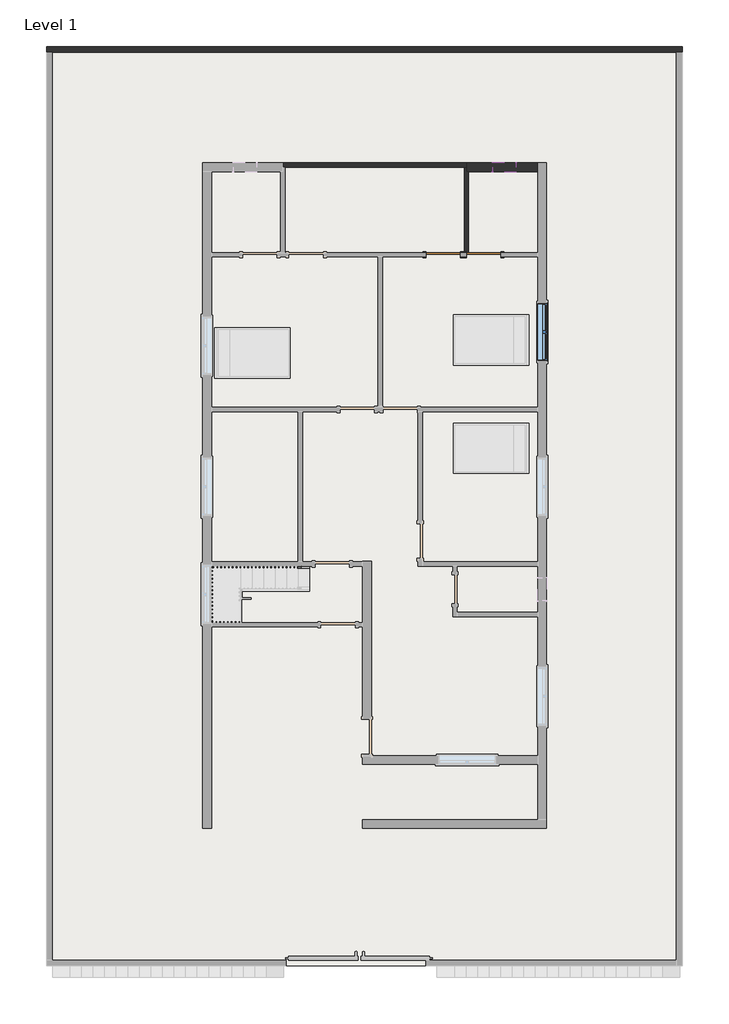
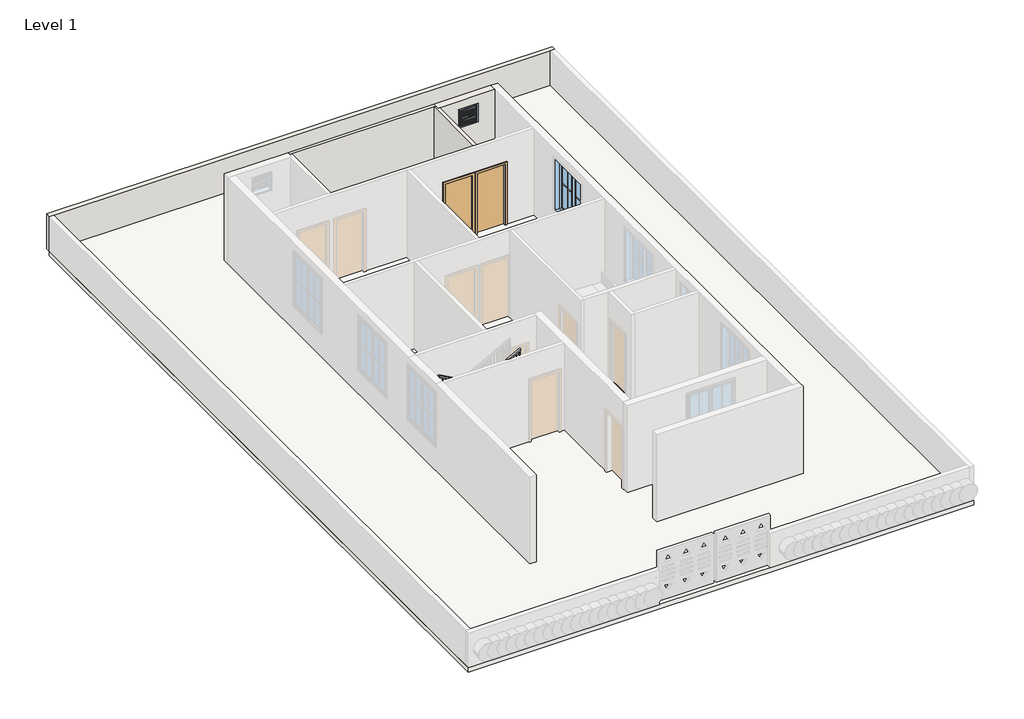
# One storey, part 2 of 3: 4 walls, 2 doors, 2 windows, 1 railing, 1 slab.
"""IFC4 building model written with IfcOpenShell, lengths in millimetres."""

from ifc_helpers import new_model, si_unit, frame, origin, origin_with_axes, place, context, project, spatial, polyline, outline, extrude, faceted_brep, transform, mapped, element, save
from components import single_flush_door_3_e5f9f3c4, single_flush_door_3_305aa2a5, window_casement_double_win_5_f93960c7, window_f2d8fef0

model = new_model("IFC4")

# Units and contexts
model_context = context("Model", 3, world=origin())
ifc_project = project(units=[si_unit("LENGTHUNIT", "METRE", prefix="MILLI")], contexts=[model_context])

# Site, building, storey
site = spatial("IfcSite", under=ifc_project)
building = spatial("IfcBuilding", under=site)
storey = spatial("IfcBuildingStorey", under=building, Name="Level 1", Elevation=0.0)

# Doors
placement = place(None, origin())
single_flush_door_3_shape = single_flush_door_3_e5f9f3c4(model_context)
element("IfcDoor", 1, ObjectType="Single-Flush : DOOR 3'", at=placement, inside=storey, context=model_context, shape_type="MappedRepresentation", body=[
    mapped(single_flush_door_3_shape, transform((555.4379845, 6040.5434309, 0.0), x_axis=(1.0, 0.0, 0.0), y_axis=(0.0, 1.0, 0.0), z_axis=(0.0, 0.0, 1.0))),
])
single_flush_door_3_2_shape = single_flush_door_3_305aa2a5(model_context)
element("IfcDoor", 2, ObjectType="Single-Flush : DOOR 3'", at=placement, inside=storey, context=model_context, shape_type="MappedRepresentation", body=[
    mapped(single_flush_door_3_2_shape, transform((1622.2379845, 6040.5434309, 0.0), x_axis=(-1.0, 0.0, 0.0), y_axis=(0.0, -1.0, 0.0), z_axis=(0.0, 0.0, 1.0))),
])

# Railing
element("IfcRailing", 3, ObjectType="Handrail - Rectangular", at=placement, inside=storey, context=model_context, shape_type="SolidModel", body=[
    faceted_brep([(-2968.8120155, -2220.8065691, 1083.7333333), (-2968.8120155, -2220.8065691, 1025.620221), (-2968.8120155, -2170.0065691, 1025.620221), (-2968.8120155, -2170.0065691, 1083.7333333), (-4797.6120155, -2220.8065691, 2099.7333333), (-4810.7756177, -2220.8065691, 2048.9333333), (-4810.7756177, -2170.0065691, 2048.9333333), (-4797.6120155, -2170.0065691, 2099.7333333), (-5508.8120155, -2220.8065691, 2099.7333333), (-5508.8120155, -2220.8065691, 2048.9333333), (-5559.6120155, -2170.0065691, 2048.9333333), (-5559.6120155, -2170.0065691, 2099.7333333), (-5508.8120155, -3624.1565691, 2099.7333333), (-5508.8120155, -3624.1565691, 2048.9333333), (-5559.6120155, -3674.9565691, 2048.9333333), (-5559.6120155, -3674.9565691, 2099.7333333), (-5102.4120155, -3624.1565691, 2099.7333333), (-5089.2484132, -3624.1565691, 2048.9333333), (-5089.2484132, -3674.9565691, 2048.9333333), (-5102.4120155, -3674.9565691, 2099.7333333), (-2968.8120155, -3624.1565691, 3285.0666667), (-2968.8120155, -3674.9565691, 3285.0666667), (-2968.8120155, -3674.9565691, 3226.9535543), (-2968.8120155, -3624.1565691, 3226.9535543)], [[[0, 1, 2, 3]], [[1, 0, 4, 5]], [[2, 1, 5, 6]], [[3, 2, 6, 7]], [[0, 3, 7, 4]], [[5, 4, 8, 9]], [[6, 5, 9, 10]], [[7, 6, 10, 11]], [[4, 7, 11, 8]], [[9, 8, 12, 13]], [[10, 9, 13, 14]], [[11, 10, 14, 15]], [[8, 11, 15, 12]], [[13, 12, 16, 17]], [[14, 13, 17, 18]], [[15, 14, 18, 19]], [[12, 15, 19, 16]], [[20, 21, 22, 23]], [[17, 16, 20, 23]], [[18, 17, 23, 22]], [[19, 18, 22, 21]], [[16, 19, 21, 20]]]),
    extrude(outline(polyline([(3218.1341099, -2984.6870155), (3207.5507765, -3003.7370155), (2201.3333333, -3003.7370155), (2201.3333333, -2984.6870155), (3218.1341099, -2984.6870155)])), frame((0.0, -3659.0815691, 0.0), z_axis=(0.0, 1.0, 0.0), x_axis=(0.0, 0.0, 1.0)), (0.0, 0.0, 1.0), 19.05),
    extrude(outline(polyline([(3161.6896654, -3086.2870155), (3151.1063321, -3105.3370155), (2201.3333333, -3105.3370155), (2201.3333333, -3086.2870155), (3161.6896654, -3086.2870155)])), frame((0.0, -3659.0815691, 0.0), z_axis=(0.0, 1.0, 0.0), x_axis=(0.0, 0.0, 1.0)), (0.0, 0.0, 1.0), 19.05),
    extrude(outline(polyline([(3105.245221, -3187.8870155), (3094.6618876, -3206.9370155), (2201.3333333, -3206.9370155), (2201.3333333, -3187.8870155), (3105.245221, -3187.8870155)])), frame((0.0, -3659.0815691, 0.0), z_axis=(0.0, 1.0, 0.0), x_axis=(0.0, 0.0, 1.0)), (0.0, 0.0, 1.0), 19.05),
    extrude(outline(polyline([(3048.8007765, -3289.4870155), (3038.2174432, -3308.5370155), (2032.0, -3308.5370155), (2032.0, -3289.4870155), (3048.8007765, -3289.4870155)])), frame((0.0, -3659.0815691, 0.0), z_axis=(0.0, 1.0, 0.0), x_axis=(0.0, 0.0, 1.0)), (0.0, 0.0, 1.0), 19.05),
    extrude(outline(polyline([(2992.3563321, -3391.0870155), (2981.7729988, -3410.1370155), (2032.0, -3410.1370155), (2032.0, -3391.0870155), (2992.3563321, -3391.0870155)])), frame((0.0, -3659.0815691, 0.0), z_axis=(0.0, 1.0, 0.0), x_axis=(0.0, 0.0, 1.0)), (0.0, 0.0, 1.0), 19.05),
    extrude(outline(polyline([(2935.9118876, -3492.6870155), (2925.3285543, -3511.7370155), (2032.0, -3511.7370155), (2032.0, -3492.6870155), (2935.9118876, -3492.6870155)])), frame((0.0, -3659.0815691, 0.0), z_axis=(0.0, 1.0, 0.0), x_axis=(0.0, 0.0, 1.0)), (0.0, 0.0, 1.0), 19.05),
    extrude(outline(polyline([(2879.4674432, -3594.2870155), (2868.8841099, -3613.3370155), (1862.6666667, -3613.3370155), (1862.6666667, -3594.2870155), (2879.4674432, -3594.2870155)])), frame((0.0, -3659.0815691, 0.0), z_axis=(0.0, 1.0, 0.0), x_axis=(0.0, 0.0, 1.0)), (0.0, 0.0, 1.0), 19.05),
    extrude(outline(polyline([(2823.0229988, -3695.8870155), (2812.4396654, -3714.9370155), (1862.6666667, -3714.9370155), (1862.6666667, -3695.8870155), (2823.0229988, -3695.8870155)])), frame((0.0, -3659.0815691, 0.0), z_axis=(0.0, 1.0, 0.0), x_axis=(0.0, 0.0, 1.0)), (0.0, 0.0, 1.0), 19.05),
    extrude(outline(polyline([(2766.5785543, -3797.4870155), (2755.995221, -3816.5370155), (1862.6666667, -3816.5370155), (1862.6666667, -3797.4870155), (2766.5785543, -3797.4870155)])), frame((0.0, -3659.0815691, 0.0), z_axis=(0.0, 1.0, 0.0), x_axis=(0.0, 0.0, 1.0)), (0.0, 0.0, 1.0), 19.05),
    extrude(outline(polyline([(2710.1341099, -3899.0870155), (2699.5507765, -3918.1370155), (1693.3333333, -3918.1370155), (1693.3333333, -3899.0870155), (2710.1341099, -3899.0870155)])), frame((0.0, -3659.0815691, 0.0), z_axis=(0.0, 1.0, 0.0), x_axis=(0.0, 0.0, 1.0)), (0.0, 0.0, 1.0), 19.05),
    extrude(outline(polyline([(2653.6896654, -4000.6870155), (2643.1063321, -4019.7370155), (1693.3333333, -4019.7370155), (1693.3333333, -4000.6870155), (2653.6896654, -4000.6870155)])), frame((0.0, -3659.0815691, 0.0), z_axis=(0.0, 1.0, 0.0), x_axis=(0.0, 0.0, 1.0)), (0.0, 0.0, 1.0), 19.05),
    extrude(outline(polyline([(2597.245221, -4102.2870155), (2586.6618876, -4121.3370155), (1693.3333333, -4121.3370155), (1693.3333333, -4102.2870155), (2597.245221, -4102.2870155)])), frame((0.0, -3659.0815691, 0.0), z_axis=(0.0, 1.0, 0.0), x_axis=(0.0, 0.0, 1.0)), (0.0, 0.0, 1.0), 19.05),
    extrude(outline(polyline([(2540.8007765, -4203.8870155), (2530.2174432, -4222.9370155), (1524.0, -4222.9370155), (1524.0, -4203.8870155), (2540.8007765, -4203.8870155)])), frame((0.0, -3659.0815691, 0.0), z_axis=(0.0, 1.0, 0.0), x_axis=(0.0, 0.0, 1.0)), (0.0, 0.0, 1.0), 19.05),
    extrude(outline(polyline([(2484.3563321, -4305.4870155), (2473.7729988, -4324.5370155), (1524.0, -4324.5370155), (1524.0, -4305.4870155), (2484.3563321, -4305.4870155)])), frame((0.0, -3659.0815691, 0.0), z_axis=(0.0, 1.0, 0.0), x_axis=(0.0, 0.0, 1.0)), (0.0, 0.0, 1.0), 19.05),
    extrude(outline(polyline([(2427.9118876, -4407.0870155), (2417.3285543, -4426.1370155), (1524.0, -4426.1370155), (1524.0, -4407.0870155), (2427.9118876, -4407.0870155)])), frame((0.0, -3659.0815691, 0.0), z_axis=(0.0, 1.0, 0.0), x_axis=(0.0, 0.0, 1.0)), (0.0, 0.0, 1.0), 19.05),
    extrude(outline(polyline([(2371.4674432, -4508.6870155), (2360.8841099, -4527.7370155), (1354.6666667, -4527.7370155), (1354.6666667, -4508.6870155), (2371.4674432, -4508.6870155)])), frame((0.0, -3659.0815691, 0.0), z_axis=(0.0, 1.0, 0.0), x_axis=(0.0, 0.0, 1.0)), (0.0, 0.0, 1.0), 19.05),
    extrude(outline(polyline([(2315.0229988, -4610.2870155), (2304.4396654, -4629.3370155), (1354.6666667, -4629.3370155), (1354.6666667, -4610.2870155), (2315.0229988, -4610.2870155)])), frame((0.0, -3659.0815691, 0.0), z_axis=(0.0, 1.0, 0.0), x_axis=(0.0, 0.0, 1.0)), (0.0, 0.0, 1.0), 19.05),
    extrude(outline(polyline([(2258.5785543, -4711.8870155), (2247.995221, -4730.9370155), (1354.6666667, -4730.9370155), (1354.6666667, -4711.8870155), (2258.5785543, -4711.8870155)])), frame((0.0, -3659.0815691, 0.0), z_axis=(0.0, 1.0, 0.0), x_axis=(0.0, 0.0, 1.0)), (0.0, 0.0, 1.0), 19.05),
    extrude(outline(polyline([(2202.1341099, -4813.4870155), (2191.5507765, -4832.5370155), (1185.3333333, -4832.5370155), (1185.3333333, -4813.4870155), (2202.1341099, -4813.4870155)])), frame((0.0, -3659.0815691, 0.0), z_axis=(0.0, 1.0, 0.0), x_axis=(0.0, 0.0, 1.0)), (0.0, 0.0, 1.0), 19.05),
    extrude(outline(polyline([(2145.6896654, -4915.0870155), (2135.1063321, -4934.1370155), (1185.3333333, -4934.1370155), (1185.3333333, -4915.0870155), (2145.6896654, -4915.0870155)])), frame((0.0, -3659.0815691, 0.0), z_axis=(0.0, 1.0, 0.0), x_axis=(0.0, 0.0, 1.0)), (0.0, 0.0, 1.0), 19.05),
    extrude(outline(polyline([(2089.245221, -5016.6870155), (2078.6618876, -5035.7370155), (1185.3333333, -5035.7370155), (1185.3333333, -5016.6870155), (2089.245221, -5016.6870155)])), frame((0.0, -3659.0815691, 0.0), z_axis=(0.0, 1.0, 0.0), x_axis=(0.0, 0.0, 1.0)), (0.0, 0.0, 1.0), 19.05),
    extrude(outline(polyline([(-5137.3370155, -3659.0815691), (-5137.3370155, -3640.0315691), (-5118.2870155, -3640.0315691), (-5118.2870155, -3659.0815691), (-5137.3370155, -3659.0815691)])), frame((0.0, 0.0, 1185.3333333), z_axis=(0.0, 0.0, 1.0), x_axis=(1.0, 0.0, 0.0)), (0.0, 0.0, 1.0), 863.6),
    extrude(outline(polyline([(-5238.9370155, -3659.0815691), (-5238.9370155, -3640.0315691), (-5219.8870155, -3640.0315691), (-5219.8870155, -3659.0815691), (-5238.9370155, -3659.0815691)])), frame((0.0, 0.0, 1185.3333333), z_axis=(0.0, 0.0, 1.0), x_axis=(1.0, 0.0, 0.0)), (0.0, 0.0, 1.0), 863.6),
    extrude(outline(polyline([(-5340.5370155, -3659.0815691), (-5340.5370155, -3640.0315691), (-5321.4870155, -3640.0315691), (-5321.4870155, -3659.0815691), (-5340.5370155, -3659.0815691)])), frame((0.0, 0.0, 1185.3333333), z_axis=(0.0, 0.0, 1.0), x_axis=(1.0, 0.0, 0.0)), (0.0, 0.0, 1.0), 863.6),
    extrude(outline(polyline([(-5442.1370155, -3659.0815691), (-5442.1370155, -3640.0315691), (-5423.0870155, -3640.0315691), (-5423.0870155, -3659.0815691), (-5442.1370155, -3659.0815691)])), frame((0.0, 0.0, 1185.3333333), z_axis=(0.0, 0.0, 1.0), x_axis=(1.0, 0.0, 0.0)), (0.0, 0.0, 1.0), 863.6),
    extrude(outline(polyline([(-5543.7370155, -3608.2815691), (-5524.6870155, -3608.2815691), (-5524.6870155, -3627.3315691), (-5543.7370155, -3627.3315691), (-5543.7370155, -3608.2815691)])), frame((0.0, 0.0, 1185.3333333), z_axis=(0.0, 0.0, 1.0), x_axis=(1.0, 0.0, 0.0)), (0.0, 0.0, 1.0), 863.6),
    extrude(outline(polyline([(-5543.7370155, -3506.6815691), (-5524.6870155, -3506.6815691), (-5524.6870155, -3525.7315691), (-5543.7370155, -3525.7315691), (-5543.7370155, -3506.6815691)])), frame((0.0, 0.0, 1185.3333333), z_axis=(0.0, 0.0, 1.0), x_axis=(1.0, 0.0, 0.0)), (0.0, 0.0, 1.0), 863.6),
    extrude(outline(polyline([(-5543.7370155, -3405.0815691), (-5524.6870155, -3405.0815691), (-5524.6870155, -3424.1315691), (-5543.7370155, -3424.1315691), (-5543.7370155, -3405.0815691)])), frame((0.0, 0.0, 1185.3333333), z_axis=(0.0, 0.0, 1.0), x_axis=(1.0, 0.0, 0.0)), (0.0, 0.0, 1.0), 863.6),
    extrude(outline(polyline([(-5543.7370155, -3303.4815691), (-5524.6870155, -3303.4815691), (-5524.6870155, -3322.5315691), (-5543.7370155, -3322.5315691), (-5543.7370155, -3303.4815691)])), frame((0.0, 0.0, 1185.3333333), z_axis=(0.0, 0.0, 1.0), x_axis=(1.0, 0.0, 0.0)), (0.0, 0.0, 1.0), 863.6),
    extrude(outline(polyline([(-5543.7370155, -3201.8815691), (-5524.6870155, -3201.8815691), (-5524.6870155, -3220.9315691), (-5543.7370155, -3220.9315691), (-5543.7370155, -3201.8815691)])), frame((0.0, 0.0, 1185.3333333), z_axis=(0.0, 0.0, 1.0), x_axis=(1.0, 0.0, 0.0)), (0.0, 0.0, 1.0), 863.6),
    extrude(outline(polyline([(-5543.7370155, -3100.2815691), (-5524.6870155, -3100.2815691), (-5524.6870155, -3119.3315691), (-5543.7370155, -3119.3315691), (-5543.7370155, -3100.2815691)])), frame((0.0, 0.0, 1185.3333333), z_axis=(0.0, 0.0, 1.0), x_axis=(1.0, 0.0, 0.0)), (0.0, 0.0, 1.0), 863.6),
    extrude(outline(polyline([(-5543.7370155, -2998.6815691), (-5524.6870155, -2998.6815691), (-5524.6870155, -3017.7315691), (-5543.7370155, -3017.7315691), (-5543.7370155, -2998.6815691)])), frame((0.0, 0.0, 1185.3333333), z_axis=(0.0, 0.0, 1.0), x_axis=(1.0, 0.0, 0.0)), (0.0, 0.0, 1.0), 863.6),
    extrude(outline(polyline([(-5543.7370155, -2897.0815691), (-5524.6870155, -2897.0815691), (-5524.6870155, -2916.1315691), (-5543.7370155, -2916.1315691), (-5543.7370155, -2897.0815691)])), frame((0.0, 0.0, 1185.3333333), z_axis=(0.0, 0.0, 1.0), x_axis=(1.0, 0.0, 0.0)), (0.0, 0.0, 1.0), 863.6),
    extrude(outline(polyline([(-5543.7370155, -2795.4815691), (-5524.6870155, -2795.4815691), (-5524.6870155, -2814.5315691), (-5543.7370155, -2814.5315691), (-5543.7370155, -2795.4815691)])), frame((0.0, 0.0, 1185.3333333), z_axis=(0.0, 0.0, 1.0), x_axis=(1.0, 0.0, 0.0)), (0.0, 0.0, 1.0), 863.6),
    extrude(outline(polyline([(-5543.7370155, -2693.8815691), (-5524.6870155, -2693.8815691), (-5524.6870155, -2712.9315691), (-5543.7370155, -2712.9315691), (-5543.7370155, -2693.8815691)])), frame((0.0, 0.0, 1185.3333333), z_axis=(0.0, 0.0, 1.0), x_axis=(1.0, 0.0, 0.0)), (0.0, 0.0, 1.0), 863.6),
    extrude(outline(polyline([(-5543.7370155, -2592.2815691), (-5524.6870155, -2592.2815691), (-5524.6870155, -2611.3315691), (-5543.7370155, -2611.3315691), (-5543.7370155, -2592.2815691)])), frame((0.0, 0.0, 1185.3333333), z_axis=(0.0, 0.0, 1.0), x_axis=(1.0, 0.0, 0.0)), (0.0, 0.0, 1.0), 863.6),
    extrude(outline(polyline([(-5543.7370155, -2490.6815691), (-5524.6870155, -2490.6815691), (-5524.6870155, -2509.7315691), (-5543.7370155, -2509.7315691), (-5543.7370155, -2490.6815691)])), frame((0.0, 0.0, 1185.3333333), z_axis=(0.0, 0.0, 1.0), x_axis=(1.0, 0.0, 0.0)), (0.0, 0.0, 1.0), 863.6),
    extrude(outline(polyline([(-5543.7370155, -2389.0815691), (-5524.6870155, -2389.0815691), (-5524.6870155, -2408.1315691), (-5543.7370155, -2408.1315691), (-5543.7370155, -2389.0815691)])), frame((0.0, 0.0, 1185.3333333), z_axis=(0.0, 0.0, 1.0), x_axis=(1.0, 0.0, 0.0)), (0.0, 0.0, 1.0), 863.6),
    extrude(outline(polyline([(-5543.7370155, -2287.4815691), (-5524.6870155, -2287.4815691), (-5524.6870155, -2306.5315691), (-5543.7370155, -2306.5315691), (-5543.7370155, -2287.4815691)])), frame((0.0, 0.0, 1185.3333333), z_axis=(0.0, 0.0, 1.0), x_axis=(1.0, 0.0, 0.0)), (0.0, 0.0, 1.0), 863.6),
    extrude(outline(polyline([(-5499.2870155, -2185.8815691), (-5499.2870155, -2204.9315691), (-5518.3370155, -2204.9315691), (-5518.3370155, -2185.8815691), (-5499.2870155, -2185.8815691)])), frame((0.0, 0.0, 1185.3333333), z_axis=(0.0, 0.0, 1.0), x_axis=(1.0, 0.0, 0.0)), (0.0, 0.0, 1.0), 863.6),
    extrude(outline(polyline([(-5397.6870155, -2185.8815691), (-5397.6870155, -2204.9315691), (-5416.7370155, -2204.9315691), (-5416.7370155, -2185.8815691), (-5397.6870155, -2185.8815691)])), frame((0.0, 0.0, 1185.3333333), z_axis=(0.0, 0.0, 1.0), x_axis=(1.0, 0.0, 0.0)), (0.0, 0.0, 1.0), 863.6),
    extrude(outline(polyline([(-5296.0870155, -2185.8815691), (-5296.0870155, -2204.9315691), (-5315.1370155, -2204.9315691), (-5315.1370155, -2185.8815691), (-5296.0870155, -2185.8815691)])), frame((0.0, 0.0, 1185.3333333), z_axis=(0.0, 0.0, 1.0), x_axis=(1.0, 0.0, 0.0)), (0.0, 0.0, 1.0), 863.6),
    extrude(outline(polyline([(-5194.4870155, -2185.8815691), (-5194.4870155, -2204.9315691), (-5213.5370155, -2204.9315691), (-5213.5370155, -2185.8815691), (-5194.4870155, -2185.8815691)])), frame((0.0, 0.0, 1185.3333333), z_axis=(0.0, 0.0, 1.0), x_axis=(1.0, 0.0, 0.0)), (0.0, 0.0, 1.0), 863.6),
    extrude(outline(polyline([(-5092.8870155, -2185.8815691), (-5092.8870155, -2204.9315691), (-5111.9370155, -2204.9315691), (-5111.9370155, -2185.8815691), (-5092.8870155, -2185.8815691)])), frame((0.0, 0.0, 1185.3333333), z_axis=(0.0, 0.0, 1.0), x_axis=(1.0, 0.0, 0.0)), (0.0, 0.0, 1.0), 863.6),
    extrude(outline(polyline([(-4991.2870155, -2185.8815691), (-4991.2870155, -2204.9315691), (-5010.3370155, -2204.9315691), (-5010.3370155, -2185.8815691), (-4991.2870155, -2185.8815691)])), frame((0.0, 0.0, 1185.3333333), z_axis=(0.0, 0.0, 1.0), x_axis=(1.0, 0.0, 0.0)), (0.0, 0.0, 1.0), 863.6),
    extrude(outline(polyline([(-4889.6870155, -2185.8815691), (-4889.6870155, -2204.9315691), (-4908.7370155, -2204.9315691), (-4908.7370155, -2185.8815691), (-4889.6870155, -2185.8815691)])), frame((0.0, 0.0, 1185.3333333), z_axis=(0.0, 0.0, 1.0), x_axis=(1.0, 0.0, 0.0)), (0.0, 0.0, 1.0), 863.6),
    extrude(outline(polyline([(2036.3285543, -4788.0870155), (2046.9118876, -4807.1370155), (1185.3333333, -4807.1370155), (1185.3333333, -4788.0870155), (2036.3285543, -4788.0870155)])), frame((0.0, -2204.9315691, 0.0), z_axis=(0.0, 1.0, 0.0), x_axis=(0.0, 0.0, 1.0)), (0.0, 0.0, 1.0), 19.05),
    extrude(outline(polyline([(1979.8841099, -4686.4870155), (1990.4674432, -4705.5370155), (1016.0, -4705.5370155), (1016.0, -4686.4870155), (1979.8841099, -4686.4870155)])), frame((0.0, -2204.9315691, 0.0), z_axis=(0.0, 1.0, 0.0), x_axis=(0.0, 0.0, 1.0)), (0.0, 0.0, 1.0), 19.05),
    extrude(outline(polyline([(1923.4396654, -4584.8870155), (1934.0229988, -4603.9370155), (1016.0, -4603.9370155), (1016.0, -4584.8870155), (1923.4396654, -4584.8870155)])), frame((0.0, -2204.9315691, 0.0), z_axis=(0.0, 1.0, 0.0), x_axis=(0.0, 0.0, 1.0)), (0.0, 0.0, 1.0), 19.05),
    extrude(outline(polyline([(1866.995221, -4483.2870155), (1877.5785543, -4502.3370155), (1016.0, -4502.3370155), (1016.0, -4483.2870155), (1866.995221, -4483.2870155)])), frame((0.0, -2204.9315691, 0.0), z_axis=(0.0, 1.0, 0.0), x_axis=(0.0, 0.0, 1.0)), (0.0, 0.0, 1.0), 19.05),
    extrude(outline(polyline([(1810.5507765, -4381.6870155), (1821.1341099, -4400.7370155), (846.6666667, -4400.7370155), (846.6666667, -4381.6870155), (1810.5507765, -4381.6870155)])), frame((0.0, -2204.9315691, 0.0), z_axis=(0.0, 1.0, 0.0), x_axis=(0.0, 0.0, 1.0)), (0.0, 0.0, 1.0), 19.05),
    extrude(outline(polyline([(1754.1063321, -4280.0870155), (1764.6896654, -4299.1370155), (846.6666667, -4299.1370155), (846.6666667, -4280.0870155), (1754.1063321, -4280.0870155)])), frame((0.0, -2204.9315691, 0.0), z_axis=(0.0, 1.0, 0.0), x_axis=(0.0, 0.0, 1.0)), (0.0, 0.0, 1.0), 19.05),
    extrude(outline(polyline([(1697.6618876, -4178.4870155), (1708.245221, -4197.5370155), (846.6666667, -4197.5370155), (846.6666667, -4178.4870155), (1697.6618876, -4178.4870155)])), frame((0.0, -2204.9315691, 0.0), z_axis=(0.0, 1.0, 0.0), x_axis=(0.0, 0.0, 1.0)), (0.0, 0.0, 1.0), 19.05),
    extrude(outline(polyline([(1641.2174432, -4076.8870155), (1651.8007765, -4095.9370155), (677.3333333, -4095.9370155), (677.3333333, -4076.8870155), (1641.2174432, -4076.8870155)])), frame((0.0, -2204.9315691, 0.0), z_axis=(0.0, 1.0, 0.0), x_axis=(0.0, 0.0, 1.0)), (0.0, 0.0, 1.0), 19.05),
    extrude(outline(polyline([(1584.7729988, -3975.2870155), (1595.3563321, -3994.3370155), (677.3333333, -3994.3370155), (677.3333333, -3975.2870155), (1584.7729988, -3975.2870155)])), frame((0.0, -2204.9315691, 0.0), z_axis=(0.0, 1.0, 0.0), x_axis=(0.0, 0.0, 1.0)), (0.0, 0.0, 1.0), 19.05),
    extrude(outline(polyline([(1528.3285543, -3873.6870155), (1538.9118876, -3892.7370155), (677.3333333, -3892.7370155), (677.3333333, -3873.6870155), (1528.3285543, -3873.6870155)])), frame((0.0, -2204.9315691, 0.0), z_axis=(0.0, 1.0, 0.0), x_axis=(0.0, 0.0, 1.0)), (0.0, 0.0, 1.0), 19.05),
    extrude(outline(polyline([(1471.8841099, -3772.0870155), (1482.4674432, -3791.1370155), (508.0, -3791.1370155), (508.0, -3772.0870155), (1471.8841099, -3772.0870155)])), frame((0.0, -2204.9315691, 0.0), z_axis=(0.0, 1.0, 0.0), x_axis=(0.0, 0.0, 1.0)), (0.0, 0.0, 1.0), 19.05),
    extrude(outline(polyline([(1415.4396654, -3670.4870155), (1426.0229988, -3689.5370155), (508.0, -3689.5370155), (508.0, -3670.4870155), (1415.4396654, -3670.4870155)])), frame((0.0, -2204.9315691, 0.0), z_axis=(0.0, 1.0, 0.0), x_axis=(0.0, 0.0, 1.0)), (0.0, 0.0, 1.0), 19.05),
    extrude(outline(polyline([(1358.995221, -3568.8870155), (1369.5785543, -3587.9370155), (508.0, -3587.9370155), (508.0, -3568.8870155), (1358.995221, -3568.8870155)])), frame((0.0, -2204.9315691, 0.0), z_axis=(0.0, 1.0, 0.0), x_axis=(0.0, 0.0, 1.0)), (0.0, 0.0, 1.0), 19.05),
    extrude(outline(polyline([(1302.5507765, -3467.2870155), (1313.1341099, -3486.3370155), (338.6666667, -3486.3370155), (338.6666667, -3467.2870155), (1302.5507765, -3467.2870155)])), frame((0.0, -2204.9315691, 0.0), z_axis=(0.0, 1.0, 0.0), x_axis=(0.0, 0.0, 1.0)), (0.0, 0.0, 1.0), 19.05),
    extrude(outline(polyline([(1246.1063321, -3365.6870155), (1256.6896654, -3384.7370155), (338.6666667, -3384.7370155), (338.6666667, -3365.6870155), (1246.1063321, -3365.6870155)])), frame((0.0, -2204.9315691, 0.0), z_axis=(0.0, 1.0, 0.0), x_axis=(0.0, 0.0, 1.0)), (0.0, 0.0, 1.0), 19.05),
    extrude(outline(polyline([(1189.6618876, -3264.0870155), (1200.245221, -3283.1370155), (338.6666667, -3283.1370155), (338.6666667, -3264.0870155), (1189.6618876, -3264.0870155)])), frame((0.0, -2204.9315691, 0.0), z_axis=(0.0, 1.0, 0.0), x_axis=(0.0, 0.0, 1.0)), (0.0, 0.0, 1.0), 19.05),
    extrude(outline(polyline([(1133.2174432, -3162.4870155), (1143.8007765, -3181.5370155), (169.3333333, -3181.5370155), (169.3333333, -3162.4870155), (1133.2174432, -3162.4870155)])), frame((0.0, -2204.9315691, 0.0), z_axis=(0.0, 1.0, 0.0), x_axis=(0.0, 0.0, 1.0)), (0.0, 0.0, 1.0), 19.05),
    extrude(outline(polyline([(1076.7729988, -3060.8870155), (1087.3563321, -3079.9370155), (169.3333333, -3079.9370155), (169.3333333, -3060.8870155), (1076.7729988, -3060.8870155)])), frame((0.0, -2204.9315691, 0.0), z_axis=(0.0, 1.0, 0.0), x_axis=(0.0, 0.0, 1.0)), (0.0, 0.0, 1.0), 19.05),
    extrude(outline(polyline([(-5543.7370155, -3640.0315691), (-5524.6870155, -3640.0315691), (-5524.6870155, -3659.0815691), (-5543.7370155, -3659.0815691), (-5543.7370155, -3640.0315691)])), frame((0.0, 0.0, 1185.3333333), z_axis=(0.0, 0.0, 1.0), x_axis=(1.0, 0.0, 0.0)), (0.0, 0.0, 1.0), 863.6),
    extrude(outline(polyline([(-5524.6870155, -2185.8815691), (-5524.6870155, -2204.9315691), (-5543.7370155, -2204.9315691), (-5543.7370155, -2185.8815691), (-5524.6870155, -2185.8815691)])), frame((0.0, 0.0, 1185.3333333), z_axis=(0.0, 0.0, 1.0), x_axis=(1.0, 0.0, 0.0)), (0.0, 0.0, 1.0), 863.6),
    extrude(outline(polyline([(3226.9535543, -2968.8120155), (3216.370221, -2987.8620155), (2201.3333333, -2987.8620155), (2201.3333333, -2968.8120155), (3226.9535543, -2968.8120155)])), frame((0.0, -3659.0815691, 0.0), z_axis=(0.0, 1.0, 0.0), x_axis=(0.0, 0.0, 1.0)), (0.0, 0.0, 1.0), 19.05),
    extrude(outline(polyline([(1025.620221, -2968.8120155), (1036.2035543, -2987.8620155), (169.3333333, -2987.8620155), (169.3333333, -2968.8120155), (1025.620221, -2968.8120155)])), frame((0.0, -2204.9315691, 0.0), z_axis=(0.0, 1.0, 0.0), x_axis=(0.0, 0.0, 1.0)), (0.0, 0.0, 1.0), 19.05),
])

# Slab
element("IfcSlab", 4, ObjectType="FLOOR 6\"", at=placement, inside=storey, context=model_context, shape_type="SweptSolid", body=[
    extrude(outline(polyline([(6853.8726148, 11374.8947978), (6853.8726148, -12704.3052022), (-9910.1273852, -12704.3052022), (-9910.1273852, 11374.8947978), (6853.8726148, 11374.8947978)])), frame((0.0, 0.0, -152.4), z_axis=(0.0, 0.0, 1.0), x_axis=(1.0, 0.0, 0.0)), (0.0, 0.0, 1.0), 152.4),
])

# Walls
element("IfcWall", 5, ObjectType="CMD 6\"", at=placement, inside=storey, context=model_context, shape_type="Brep", body=[
    faceted_brep([(-9910.1273852, 11374.8947978, 0.0), (-9757.7273852, 11374.8947978, 0.0), (6701.4726148, 11374.8947978, 0.0), (6853.8726148, 11374.8947978, 0.0), (6853.8726148, 11374.8947978, 1219.2), (6701.4726148, 11374.8947978, 1219.2), (-9757.7273852, 11374.8947978, 1219.2), (-9910.1273852, 11374.8947978, 1219.2), (-9910.1273852, 11527.2947978, 0.0), (-9910.1273852, 11527.2947978, 1219.2), (6853.8726148, 11527.2947978, 1219.2), (6853.8726148, 11527.2947978, 0.0)], [[[0, 1, 2, 3, 4, 5, 6, 7]], [[8, 9, 10, 11]], [[3, 2, 1, 0, 8, 11]], [[7, 6, 5, 4, 10, 9]], [[4, 3, 11, 10]], [[0, 7, 9, 8]]]),
])
element("IfcWall", 6, ObjectType="WALL 4.5\"", at=placement, inside=storey, context=model_context, shape_type="Brep", body=[
    faceted_brep([(-3673.6620155, 8345.5934309, 0.0), (-3616.5120155, 8345.5934309, 0.0), (1107.8879845, 8345.5934309, 0.0), (1165.0379845, 8345.5934309, 0.0), (1165.0379845, 8345.5934309, 3048.0), (1107.8879845, 8345.5934309, 3048.0), (-3616.5120155, 8345.5934309, 3048.0), (-3673.6620155, 8345.5934309, 3048.0), (-3673.6620155, 8459.8934309, 0.0), (-3673.6620155, 8459.8934309, 3048.0), (1165.0379845, 8459.8934309, 3048.0), (1165.0379845, 8459.8934309, 0.0)], [[[0, 1, 2, 3, 4, 5, 6, 7]], [[8, 9, 10, 11]], [[3, 2, 1, 0, 8, 11]], [[4, 3, 11, 10]], [[0, 7, 9, 8]], [[7, 6, 5, 4, 10, 9]]]),
])
element("IfcWall", 7, ObjectType="WALL 4.5\"", at=placement, inside=storey, context=model_context, shape_type="SweptSolid", body=[
    extrude(outline(polyline([(1107.8879845, 6097.6934309), (1107.8879845, 8345.5934309), (1165.0379845, 8345.5934309), (1165.0379845, 8231.2934309), (1222.1879845, 8231.2934309), (1222.1879845, 6097.6934309), (1107.8879845, 6097.6934309)])), origin_with_axes(), (0.0, 0.0, 1.0), 3048.0),
])
element("IfcWall", 8, ObjectType="WALL 9\"", at=placement, inside=storey, context=model_context, shape_type="Brep", body=[
    faceted_brep([(3050.9879845, 8459.8934309, 0.0), (1165.0379845, 8459.8934309, 0.0), (1165.0379845, 8459.8934309, 3048.0), (3050.9879845, 8459.8934309, 3048.0), (2469.9629845, 8459.8934309, 2743.2), (1860.3629845, 8459.8934309, 2743.2), (1860.3629845, 8459.8934309, 2133.6), (2469.9629845, 8459.8934309, 2133.6), (3050.9879845, 8231.2934309, 0.0), (3050.9879845, 8231.2934309, 3048.0), (1222.1879845, 8231.2934309, 3048.0), (1165.0379845, 8231.2934309, 3048.0), (1165.0379845, 8231.2934309, 0.0), (1222.1879845, 8231.2934309, 0.0), (2469.9629845, 8231.2934309, 2743.2), (2469.9629845, 8231.2934309, 2133.6), (1860.3629845, 8231.2934309, 2133.6), (1860.3629845, 8231.2934309, 2743.2), (1165.0379845, 8345.5934309, 0.0), (1165.0379845, 8345.5934309, 3048.0)], [[[0, 1, 2, 3], [4, 5, 6, 7]], [[8, 9, 10, 11, 12, 13], [14, 15, 16, 17]], [[1, 0, 8, 13, 12, 18]], [[2, 1, 18, 12, 11, 19]], [[0, 3, 9, 8]], [[15, 14, 4, 7]], [[16, 15, 7, 6]], [[17, 16, 6, 5]], [[14, 17, 5, 4]], [[3, 2, 19, 11, 10, 9]]]),
])

# Windows
window_casement_double_win_5_shape = window_casement_double_win_5_f93960c7(model_context)
element("IfcWindow", 9, ObjectType="Window-Casement-Double : WIN 5'", at=placement, inside=storey, context=model_context, shape_type="MappedRepresentation", body=[
    mapped(window_casement_double_win_5_shape, transform((3165.2879845, 4002.1934309, 0.0), x_axis=(0.0, -1.0, 0.0), y_axis=(1.0, 0.0, 0.0), z_axis=(0.0, 0.0, 1.0))),
])
window_shape = window_f2d8fef0(model_context)
element("IfcWindow", 10, ObjectType="Window-Louvers : 24\" x 24\"", at=placement, inside=storey, context=model_context, shape_type="MappedRepresentation", body=[
    mapped(window_shape, transform((2165.1629845, 8339.2434309, 1219.2), x_axis=(-1.0, 0.0, 0.0), y_axis=(0.0, -1.0, 0.0), z_axis=(0.0, 0.0, 1.0))),
])

save(model, "model.ifc")

# Revit data of these elements
# Type "Single-Flush : DOOR 3'"
#   Type Mark = "9"
#   Construction Type Id = "MDOOR"
#   Assembly Code = "C1020"
#   Analytic Construction = "Metal"
#   Thickness = 0' - 2"
#   Heat Transfer Coefficient (U) = 0.651978 BTU/(h·ft²·°F)
#   Height = 7' - 0"
#   Trim Projection Ext = 0' - 1"
#   Trim Projection Int = 0' - 1"
#   Trim Width = 0' - 3"
#   Width = 3' - 0"
#   Define Thermal Properties by = 1
#   Door Material = Door - Panel
#   Frame Material = Door - Frame
#   Visual Light Transmittance = 0
#   Solar Heat Gain Coefficient = 0
#   Function = (empty or 0)
#   Wall Closure = (empty or 0)
# Type "Handrail - Rectangular"
#   Assembly Code = "C2010400"
#   built-in parameter 1008612 = 0.0416667 (stored number, unit not read)
#   built-in parameter 1008611 = 0.0416667 (stored number, unit not read)
#   built-in parameter 1008609 = 0.333333 (stored number, unit not read)
#   built-in parameter 1008604 = 0.166667 (stored number, unit not read)
#   built-in parameter 1008603 = 0.166667 (stored number, unit not read)
#   Railing Height = 3' - 0"
#   built-in parameter 1008630 = 2
#   built-in parameter 1008610 = 2
#   built-in parameter 1008618 = Baluster - Square : 3/4"
# Type "FLOOR 6\""
#   Assembly Code = "B1010"
#   Function = 0
#   Layers, outside or top first: 0' - 6" no material (function 1)
# Type "CMD 6\""
#   Assembly Code = "B2010"
#   Layers, outside or top first: 0' - 6" no material (function 1)
# Type "WALL 4.5\""
#   Assembly Code = "B2010"
#   Layers, outside or top first: 0' - 4 1/2" no material (function 1)
# Type "WALL 9\""
#   Assembly Code = "B2010"
#   Layers, outside or top first: 0' - 9" no material (function 1)
# Type "Window-Casement-Double : WIN 5'"
#   Type Mark = "18"
#   Fire Rating = "0.5h"
#   Assembly Code = "B2020100"
#   Analytic Construction = "Double glazing - domestic"
#   Frame Extension [instance default] = 0' - 0 1/4"
#   Window Inset [instance default] = 0' - 0"
#   Wall Thickness [instance default] = 0' - 6"
#   Interior Wall Closure [instance default] = 0' - 2 1/4"
#   Half Width = 2' - 6"
#   Visual Light Transmittance = 0.81
#   Thermal Resistance (R) = 1.8146 (h·ft²·°F)/BTU
#   Solar Heat Gain Coefficient = 0.76
#   Rough Width = 5' - 0 1/2"
#   Rough Height = 6' - 0 1/2"
#   Height = 6' - 0"
#   Heat Transfer Coefficient (U) = 0.5511 BTU/(h·ft²·°F)
#   Exterior Wall Closure [instance default] = 0' - 1 1/4"
#   Extension Jamb [instance default] = 0' - 2 1/4"
#   Default Sill Height = 3' - 0"
#   Width = 5' - 0"
#   Muntin Visibility = yes
#   Interior Trim Visibility [instance default] = yes
#   Exterior Trim Visibility [instance default] = yes
#   Extension Jamb Visibility [instance default] = yes
#   Interior Trim Material = Wood - Stained
#   Muntin Pattern = Muntin Pattern_2x2 : Muntin Pattern_2x2
#   Interior Trim = Trim-Window-Interior-Flat : Picture Frame
#   Interior Frame Material = Wood - Stained
#   Glass Panel Material = Glass
#   Exterior Trim Material = Clad - White
#   Exterior Trim = Trim-Window-Exterior-Flat : with Sill
#   Exterior Frame Material = Clad - White
#   Wall Closure = (empty or 0)
# Type "Window-Louvers : 24\" x 24\""
#   Type Mark = "19"
#   Construction Type Id = "GSP4R"
#   Assembly Code = "B20"
#   Analytic Construction = "1/8 in Pilkington single glazing"
#   Visual Light Transmittance = 0.9
#   Thermal Resistance (R) = 1.53941 (h·ft²·°F)/BTU
#   Solar Heat Gain Coefficient = 0.78
#   Max Height = 1' - 11.74264"
#   Height = 2' - 0"
#   Heat Transfer Coefficient (U) = 0.6496 BTU/(h·ft²·°F)
#   Blade Width [instance default] = 1' - 10 1/2"
#   Blade Vertical Thickness = 0' - 0.35355"
#   Blade Thickness = 0' - 0 1/4"
#   Blade Spacing = 0' - 1 1/2"
#   Blade Height = 0' - 1.85355"
#   Blade Depth = 0' - 3"
#   Blade Angle = 45.00°
#   Default Sill Height = 3' - 0"
#   Trim Projection_Exterior = 0' - 0 1/2"
#   Trim Projection_Interior = 0' - 0 1/2"
#   Trim Width_Exterior = 0' - 1 1/2"
#   Trim Width_Interior = 0' - 1 1/2"
#   Width = 2' - 0"
#   Max Blade Count = 12
#   Define Thermal Properties by = 1
#   Blade Count = 12
#   Frame Material = Birch
#   Louver Material = Birch
#   Trim Exterior Material = Birch
#   Trim Interior Material = Birch
#   Wall Closure = (empty or 0)
# Elements 1, 2 (IfcDoor, "Single-Flush : DOOR 3'")
#   Phase Created = New Construction
#   Materials on its faces: "Door - Frame", "Door - Panel"
# Element 3 (IfcRailing, "Handrail - Rectangular")
#   Phase Created = New Construction
# Element 4 (IfcSlab, "FLOOR 6\"")
#   Height Offset From Level = 0' - 0"
#   Phase Created = New Construction
#   Materials on its faces: "Default Floor", "Birch"
# Element 5 (IfcWall, "CMD 6\"")
#   Top Offset = 0' - 0"
#   Base Offset = 0' - 0"
#   Unconnected Height = 4' - 0"
#   wall height = 4' - 0"
#   Phase Created = New Construction
#   Base Constraint = Level 1
#   Materials on its faces: "Copper", "Default Wall"
# Element 6 (IfcWall, "WALL 4.5\"")
#   Top Offset = 0' - 0"
#   Base Offset = 0' - 0"
#   Unconnected Height = 10' - 0"
#   wall height = 10' - 0"
#   Phase Created = New Construction
#   Base Constraint = Level 1
#   Materials on its faces: "Default Wall", "Brick, Common"
# Element 7 (IfcWall, "WALL 4.5\"")
#   Top Offset = 0' - 0"
#   Base Offset = 0' - 0"
#   Unconnected Height = 10' - 0"
#   wall height = 10' - 0"
#   Phase Created = New Construction
#   Base Constraint = Level 1
#   Materials on its faces: "Default Wall"
# Element 8 (IfcWall, "WALL 9\"")
#   Top Offset = 0' - 0"
#   Base Offset = 0' - 0"
#   Unconnected Height = 10' - 0"
#   wall height = 10' - 0"
#   Phase Created = New Construction
#   Base Constraint = Level 1
#   Materials on its faces: "Default Wall", "Brick, Common"
# Element 9 (IfcWindow, "Window-Casement-Double : WIN 5'")
#   Mark = "2"
#   Window Inset = 0' - 0"
#   Interior Wall Closure = 0' - 2 1/4"
#   Frame Extension = 0' - 0 1/4"
#   Exterior Wall Closure = 0' - 1 1/4"
#   Interior Trim Visibility = yes
#   Exterior Trim Visibility = yes
#   Phase Created = New Construction
#   Materials on its faces: "Wood - Stained", "Glass", "Clad - White"
# Element 10 (IfcWindow, "Window-Louvers : 24\" x 24\"")
#   Mark = "9"
#   Blade Width = 1' - 10 1/2"
#   Phase Created = New Construction
#   Materials on its faces: "Birch"
# Materials
#   "Door - Panel": class "Wood", colour RGB 210 159 95, transparency 0, Cost = 0
#   "Door - Frame": colour RGB 118 70 51, transparency 0, Cost = 0
#   "Wood - Stained": class "Wood", colour RGB 224 178 126, transparency 0, Cost = 0
#   "Glass": class "Glass", colour RGB 0 128 192, transparency 0.75, Description = "Soda Lime Glass", Cost = 0
#   "Clad - White": class "Wood", colour RGB 242 242 238, transparency 0, Cost = 0
#   "Birch": class "Wood", colour RGB 224 178 126, transparency 0, Description = "Betula Alleghaniensis", Cost = 0
#   "Default Floor": colour RGB 128 128 128, transparency 0, Cost = 0
#   "Copper": class "Metal", colour RGB 0 0 0, transparency 0, Description = "Copper, matte finish", Cost = 0
#   "Default Wall": colour RGB 128 128 128, transparency 0, Cost = 0
#   "Brick, Common": class "Masonry", colour RGB 170 98 104, transparency 0, Description = "Common brick", Cost = 0
